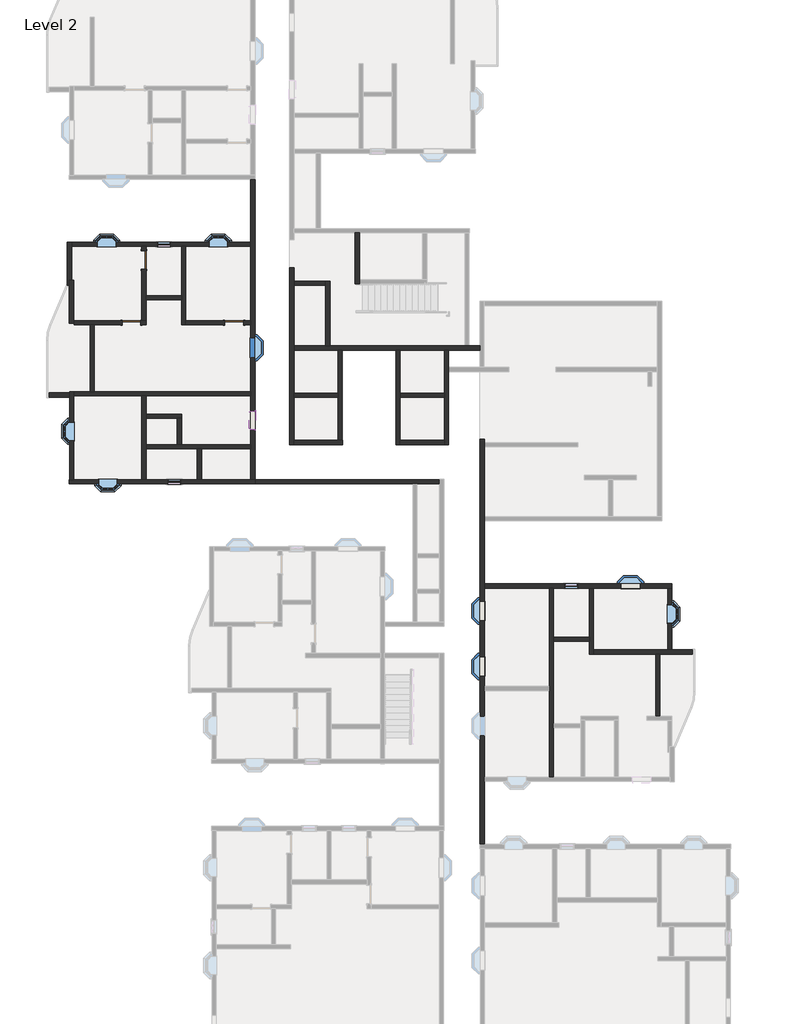
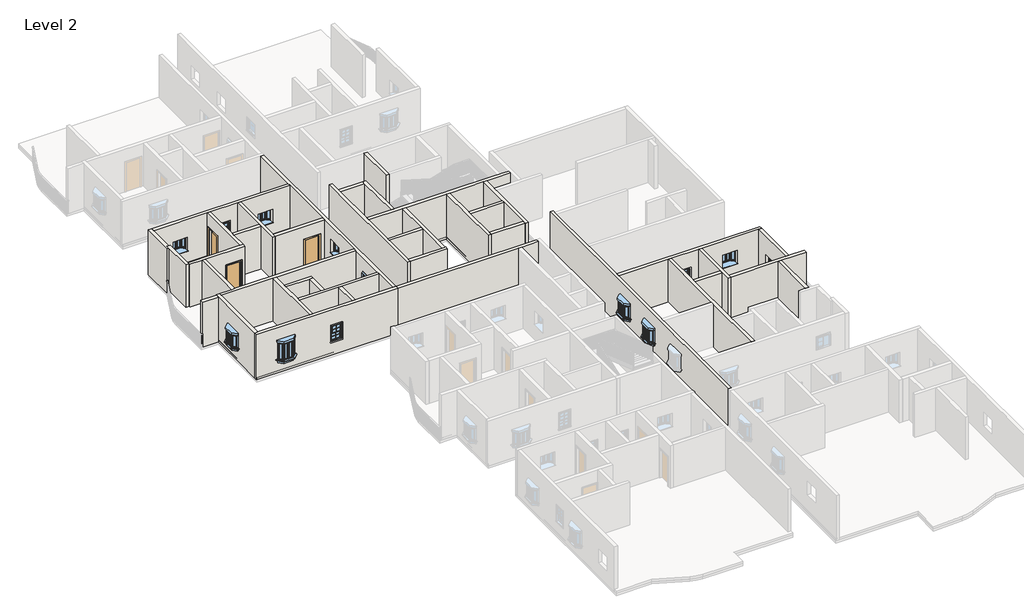
# One storey, part 3 of 14: 40 walls, 13 windows, 3 doors.
"""IFC4 building model written with IfcOpenShell, lengths in millimetres."""

from ifc_helpers import new_model, si_unit, frame, origin, place, context, project, spatial, polyline, outline, extrude, faceted_brep, transform, mapped, element, save
from components import door_54dd4da4, window_910x1210mm_154f9356, window_910x910mm_67ef725a, window_8debb0fa, windows_sgl_w_glazing_bars_910x910mm_256712d0

model = new_model("IFC4")

# Units and contexts
model_context = context("Model", 3, world=origin())
ifc_project = project(units=[si_unit("LENGTHUNIT", "METRE", prefix="MILLI")], contexts=[model_context])

# Site, building, storey
site = spatial("IfcSite", under=ifc_project)
building = spatial("IfcBuilding", under=site)
storey = spatial("IfcBuildingStorey", under=building, Name="Level 2", Elevation=3048.0)

# Doors
placement = place(None, origin())
door_shape = door_54dd4da4(model_context)
element("IfcDoor", 1, ObjectType="Single-Flush : 36\" x 84\"", at=placement, inside=storey, context=model_context, shape_type="MappedRepresentation", body=[
    mapped(door_shape, transform((-11210.3891351, 10605.7083494, 3048.0), x_axis=(1.0, 0.0, 0.0), y_axis=(0.0, 1.0, 0.0), z_axis=(0.0, 0.0, 1.0))),
])
element("IfcDoor", 2, ObjectType="Single-Flush : 36\" x 84\"", at=placement, inside=storey, context=model_context, shape_type="MappedRepresentation", body=[
    mapped(door_shape, transform((-15610.9391351, 13672.7583494, 3048.0), x_axis=(0.0, -1.0, 0.0), y_axis=(1.0, 0.0, 0.0), z_axis=(0.0, 0.0, 1.0))),
])
element("IfcDoor", 3, ObjectType="Single-Flush : 36\" x 84\"", at=placement, inside=storey, context=model_context, shape_type="MappedRepresentation", body=[
    mapped(door_shape, transform((-16220.5391351, 10605.7083494, 3048.0), x_axis=(1.0, 0.0, 0.0), y_axis=(0.0, 1.0, 0.0), z_axis=(0.0, 0.0, 1.0))),
])

# Walls
element("IfcWall", 4, ObjectType="4.5\" p", at=placement, inside=storey, context=model_context, shape_type="Brep", body=[
    faceted_brep([(-15509.3391351, 4456.3873146, 3048.0), (-13007.4391351, 4456.3873146, 3048.0), (-12804.2391351, 4456.3873146, 3048.0), (-10397.5891351, 4456.3873146, 3048.0), (-10397.5891351, 4456.3873146, 6096.0), (-12804.2391351, 4456.3873146, 6096.0), (-13007.4391351, 4456.3873146, 6096.0), (-15509.3391351, 4456.3873146, 6096.0), (-15509.3391351, 4659.5873146, 3048.0), (-15509.3391351, 4659.5873146, 6096.0), (-13985.3391351, 4659.5873146, 6096.0), (-13782.1391351, 4659.5873146, 6096.0), (-10397.5891351, 4659.5873146, 6096.0), (-10397.5891351, 4659.5873146, 3048.0), (-13782.1391351, 4659.5873146, 3048.0), (-13985.3391351, 4659.5873146, 3048.0)], [[[0, 1, 2, 3, 4, 5, 6, 7]], [[8, 9, 10, 11, 12, 13, 14, 15]], [[3, 2, 1, 0, 8, 15, 14, 13]], [[7, 6, 5, 4, 12, 11, 10, 9]], [[4, 3, 13, 12]], [[0, 7, 9, 8]]]),
])
element("IfcWall", 5, ObjectType="4.5\" p", at=placement, inside=storey, context=model_context, shape_type="SweptSolid", body=[
    extrude(outline(polyline([(-13007.4391351, 2953.9583494), (-13007.4391351, 4456.3873146), (-12804.2391351, 4456.3873146), (-12804.2391351, 2953.9583494), (-13007.4391351, 2953.9583494)])), frame((0.0, 0.0, 3048.0), z_axis=(0.0, 0.0, 1.0), x_axis=(1.0, 0.0, 0.0)), (0.0, 0.0, 1.0), 3048.0),
])
element("IfcWall", 6, ObjectType="4.5\" p", at=placement, inside=storey, context=model_context, shape_type="Brep", body=[
    faceted_brep([(-15509.3391351, 5953.2975261, 3048.0), (-13985.3391351, 5953.2975261, 3048.0), (-13782.1391351, 5953.2975261, 3048.0), (-13782.1391351, 5953.2975261, 6096.0), (-13985.3391351, 5953.2975261, 6096.0), (-15509.3391351, 5953.2975261, 6096.0), (-15509.3391351, 6156.4975261, 3048.0), (-15509.3391351, 6156.4975261, 6096.0), (-13782.1391351, 6156.4975261, 6096.0), (-13782.1391351, 6156.4975261, 3048.0)], [[[0, 1, 2, 3, 4, 5]], [[6, 7, 8, 9]], [[2, 1, 0, 6, 9]], [[5, 4, 3, 8, 7]], [[0, 5, 7, 6]], [[3, 2, 9, 8]]]),
])
element("IfcWall", 7, ObjectType="4.5\" p", at=placement, inside=storey, context=model_context, shape_type="SweptSolid", body=[
    extrude(outline(polyline([(-13985.3391351, 4659.5873146), (-13985.3391351, 5953.2975261), (-13782.1391351, 5953.2975261), (-13782.1391351, 4659.5873146), (-13985.3391351, 4659.5873146)])), frame((0.0, 0.0, 3048.0), z_axis=(0.0, 0.0, 1.0), x_axis=(1.0, 0.0, 0.0)), (0.0, 0.0, 1.0), 3048.0),
])
element("IfcWall", 8, ObjectType="4.5\" p", at=placement, inside=storey, context=model_context, shape_type="Brep", body=[
    faceted_brep([(-15712.5391351, 13215.5583494, 5181.6), (-15712.5391351, 13215.5583494, 3048.0), (-15712.5391351, 10707.3083494, 3048.0), (-15712.5391351, 10707.3083494, 6096.0), (-15712.5391351, 14333.1583494, 6096.0), (-15712.5391351, 14333.1583494, 3048.0), (-15712.5391351, 14129.9583494, 3048.0), (-15712.5391351, 14129.9583494, 5181.6), (-15509.3391351, 10707.3083494, 3048.0), (-15509.3391351, 11723.3083494, 3048.0), (-15509.3391351, 11926.5083494, 3048.0), (-15509.3391351, 13215.5583494, 3048.0), (-15509.3391351, 13215.5583494, 5181.6), (-15509.3391351, 14129.9583494, 5181.6), (-15509.3391351, 14129.9583494, 3048.0), (-15509.3391351, 14333.1583494, 3048.0), (-15509.3391351, 14333.1583494, 6096.0), (-15509.3391351, 11926.5083494, 6096.0), (-15509.3391351, 11723.3083494, 6096.0), (-15509.3391351, 10707.3083494, 6096.0)], [[[0, 1, 2, 3, 4, 5, 6, 7]], [[8, 9, 10, 11, 12, 13, 14, 15, 16, 17, 18, 19]], [[6, 5, 15, 14]], [[2, 1, 11, 10, 9, 8]], [[4, 3, 19, 18, 17, 16]], [[3, 2, 8, 19]], [[5, 4, 16, 15]], [[12, 11, 1, 0]], [[13, 12, 0, 7]], [[14, 13, 7, 6]]]),
])
element("IfcWall", 9, ObjectType="4.5\" p", at=placement, inside=storey, context=model_context, shape_type="Brep", body=[
    faceted_brep([(-13769.4391351, 14333.1583494, 3048.0), (-13769.4391351, 11926.5083494, 3048.0), (-13769.4391351, 11723.3083494, 3048.0), (-13769.4391351, 10504.1083494, 3048.0), (-13769.4391351, 10504.1083494, 6096.0), (-13769.4391351, 11723.3083494, 6096.0), (-13769.4391351, 11926.5083494, 6096.0), (-13769.4391351, 14333.1583494, 6096.0), (-13566.2391351, 14333.1583494, 3048.0), (-13566.2391351, 14333.1583494, 6096.0), (-13566.2391351, 10707.3083494, 6096.0), (-13566.2391351, 10504.1083494, 6096.0), (-13566.2391351, 10504.1083494, 3048.0), (-13566.2391351, 10707.3083494, 3048.0)], [[[0, 1, 2, 3, 4, 5, 6, 7]], [[8, 9, 10, 11, 12, 13]], [[3, 2, 1, 0, 8, 13, 12]], [[7, 6, 5, 4, 11, 10, 9]], [[0, 7, 9, 8]], [[4, 3, 12, 11]]]),
])
element("IfcWall", 10, ObjectType="4.5\" p", at=placement, inside=storey, context=model_context, shape_type="SweptSolid", body=[
    extrude(outline(polyline([(5181.6, -10753.1891351), (3048.0, -10753.1891351), (3048.0, -10397.5891351), (6096.0, -10397.5891351), (6096.0, -13566.2391351), (3048.0, -13566.2391351), (3048.0, -11667.5891351), (5181.6, -11667.5891351), (5181.6, -10753.1891351)])), frame((0.0, 10504.1083494, 0.0), z_axis=(0.0, 1.0, 0.0), x_axis=(0.0, 0.0, 1.0)), (0.0, 0.0, 1.0), 203.2),
])
element("IfcWall", 11, ObjectType="4.5\" p", at=placement, inside=storey, context=model_context, shape_type="SweptSolid", body=[
    extrude(outline(polyline([(-13769.4391351, 11723.3083494), (-15509.3391351, 11723.3083494), (-15509.3391351, 11926.5083494), (-13769.4391351, 11926.5083494), (-13769.4391351, 11723.3083494)])), frame((0.0, 0.0, 3048.0), z_axis=(0.0, 0.0, 1.0), x_axis=(1.0, 0.0, 0.0)), (0.0, 0.0, 1.0), 3048.0),
])
element("IfcWall", 12, ObjectType="4.5\" p", at=placement, inside=storey, context=model_context, shape_type="SweptSolid", body=[
    extrude(outline(polyline([(-6739.9891351, 12429.8715905), (-8289.3891351, 12429.8715905), (-8289.3891351, 12633.0715905), (-6739.9891351, 12633.0715905), (-6739.9891351, 12429.8715905)])), frame((0.0, 0.0, 3048.0), z_axis=(0.0, 0.0, 1.0), x_axis=(1.0, 0.0, 0.0)), (0.0, 0.0, 1.0), 3048.0),
])
element("IfcWall", 13, ObjectType="4.5\" p", at=placement, inside=storey, context=model_context, shape_type="SweptSolid", body=[
    extrude(outline(polyline([(-6130.3891351, 6970.2449943), (-8289.3891351, 6970.2449943), (-8289.3891351, 7173.4449943), (-6130.3891351, 7173.4449943), (-6130.3891351, 6970.2449943)])), frame((0.0, 0.0, 3048.0), z_axis=(0.0, 0.0, 1.0), x_axis=(1.0, 0.0, 0.0)), (0.0, 0.0, 1.0), 3048.0),
])
element("IfcWall", 14, ObjectType="4.5\" p", at=placement, inside=storey, context=model_context, shape_type="SweptSolid", body=[
    extrude(outline(polyline([(-948.7891351, 6970.2449943), (-3107.7891351, 6970.2449943), (-3107.7891351, 7173.4449943), (-948.7891351, 7173.4449943), (-948.7891351, 6970.2449943)])), frame((0.0, 0.0, 3048.0), z_axis=(0.0, 0.0, 1.0), x_axis=(1.0, 0.0, 0.0)), (0.0, 0.0, 1.0), 3048.0),
])
element("IfcWall", 15, ObjectType="4.5\" p", at=placement, inside=storey, context=model_context, shape_type="Brep", body=[
    faceted_brep([(-5298.5391351, 14988.9215905, 3048.0), (-5298.5391351, 12506.0715905, 3048.0), (-5298.5391351, 12506.0715905, 6096.0), (-5298.5391351, 14988.9215905, 6096.0), (-5095.3391351, 14988.9215905, 3048.0), (-5095.3391351, 14988.9215905, 6096.0), (-5095.3391351, 12709.2715905, 6096.0), (-5095.3391351, 12506.0715905, 6096.0), (-5095.3391351, 12506.0715905, 3048.0), (-5095.3391351, 12709.2715905, 3048.0)], [[[0, 1, 2, 3]], [[4, 5, 6, 7, 8, 9]], [[1, 0, 4, 9, 8]], [[3, 2, 7, 6, 5]], [[0, 3, 5, 4]], [[2, 1, 8, 7]]]),
])
element("IfcWall", 16, ObjectType="4.5\" p", at=placement, inside=storey, context=model_context, shape_type="SweptSolid", body=[
    extrude(outline(polyline([(-948.7891351, 4665.1949943), (-3107.7891351, 4665.1949943), (-3107.7891351, 4868.3949943), (-948.7891351, 4868.3949943), (-948.7891351, 4665.1949943)])), frame((0.0, 0.0, 3048.0), z_axis=(0.0, 0.0, 1.0), x_axis=(1.0, 0.0, 0.0)), (0.0, 0.0, 1.0), 3048.0),
])
element("IfcWall", 17, ObjectType="4.5\" p", at=placement, inside=storey, context=model_context, shape_type="Brep", body=[
    faceted_brep([(4184.4880523, -2336.4042694, 3048.0), (4184.4880523, -7130.6542694, 3048.0), (4184.4880523, -7333.8542694, 3048.0), (4184.4880523, -11556.6042694, 3048.0), (4184.4880523, -11556.6042694, 6096.0), (4184.4880523, -7333.8542694, 6096.0), (4184.4880523, -7130.6542694, 6096.0), (4184.4880523, -2336.4042694, 6096.0), (4387.6880523, -2336.4042694, 3048.0), (4387.6880523, -2336.4042694, 6096.0), (4387.6880523, -4736.7042694, 6096.0), (4387.6880523, -4939.9042694, 6096.0), (4387.6880523, -8959.4542694, 6096.0), (4387.6880523, -9162.6542694, 6096.0), (4387.6880523, -11556.6042694, 6096.0), (4387.6880523, -11556.6042694, 3048.0), (4387.6880523, -9162.6542694, 3048.0), (4387.6880523, -8959.4542694, 3048.0), (4387.6880523, -4939.9042694, 3048.0), (4387.6880523, -4736.7042694, 3048.0)], [[[0, 1, 2, 3, 4, 5, 6, 7]], [[8, 9, 10, 11, 12, 13, 14, 15, 16, 17, 18, 19]], [[3, 2, 1, 0, 8, 19, 18, 17, 16, 15]], [[7, 6, 5, 4, 14, 13, 12, 11, 10, 9]], [[4, 3, 15, 14]], [[0, 7, 9, 8]]]),
])
element("IfcWall", 18, ObjectType="4.5\" p", at=placement, inside=storey, context=model_context, shape_type="Brep", body=[
    faceted_brep([(803.8108649, 4915.2957306, 3048.0), (803.8108649, -14845.9042694, 3048.0), (803.8108649, -14845.9042694, 6096.0), (803.8108649, 4915.2957306, 6096.0), (803.8108649, -9516.0542694, 5158.0), (803.8108649, -9516.0542694, 4248.0), (803.8108649, -8606.0542694, 4248.0), (803.8108649, -8606.0542694, 5158.0), (803.8108649, -3909.0042694, 5158.0), (803.8108649, -3909.0042694, 4248.0), (803.8108649, -2999.0042694, 4248.0), (803.8108649, -2999.0042694, 5158.0), (803.8108649, -6620.4542694, 5158.0), (803.8108649, -6620.4542694, 4248.0), (803.8108649, -5710.4542694, 4248.0), (803.8108649, -5710.4542694, 5158.0), (1007.0108649, 4915.2957306, 3048.0), (1007.0108649, 4915.2957306, 6096.0), (1007.0108649, 4754.0949943, 6096.0), (1007.0108649, 4550.8949943, 6096.0), (1007.0108649, 1143.3957306, 6096.0), (1007.0108649, 940.1957306, 6096.0), (1007.0108649, -2133.2042694, 6096.0), (1007.0108649, -2336.4042694, 6096.0), (1007.0108649, -7130.6542694, 6096.0), (1007.0108649, -7333.8542694, 6096.0), (1007.0108649, -11556.6042694, 6096.0), (1007.0108649, -11759.8042694, 6096.0), (1007.0108649, -14845.9042694, 6096.0), (1007.0108649, -14845.9042694, 3048.0), (1007.0108649, -11759.8042694, 3048.0), (1007.0108649, -11556.6042694, 3048.0), (1007.0108649, -7333.8542694, 3048.0), (1007.0108649, -7130.6542694, 3048.0), (1007.0108649, -2336.4042694, 3048.0), (1007.0108649, -2133.2042694, 3048.0), (1007.0108649, 940.1957306, 3048.0), (1007.0108649, 1143.3957306, 3048.0), (1007.0108649, 4550.8949943, 3048.0), (1007.0108649, 4754.0949943, 3048.0), (1007.0108649, -9516.0542694, 5158.0), (1007.0108649, -8606.0542694, 5158.0), (1007.0108649, -8606.0542694, 4248.0), (1007.0108649, -9516.0542694, 4248.0), (1007.0108649, -3909.0042694, 5158.0), (1007.0108649, -2999.0042694, 5158.0), (1007.0108649, -2999.0042694, 4248.0), (1007.0108649, -3909.0042694, 4248.0), (1007.0108649, -6620.4542694, 5158.0), (1007.0108649, -5710.4542694, 5158.0), (1007.0108649, -5710.4542694, 4248.0), (1007.0108649, -6620.4542694, 4248.0)], [[[0, 1, 2, 3], [4, 5, 6, 7], [8, 9, 10, 11], [12, 13, 14, 15]], [[16, 17, 18, 19, 20, 21, 22, 23, 24, 25, 26, 27, 28, 29, 30, 31, 32, 33, 34, 35, 36, 37, 38, 39], [40, 41, 42, 43], [44, 45, 46, 47], [48, 49, 50, 51]], [[1, 0, 16, 39, 38, 37, 36, 35, 34, 33, 32, 31, 30, 29]], [[3, 2, 28, 27, 26, 25, 24, 23, 22, 21, 20, 19, 18, 17]], [[0, 3, 17, 16]], [[2, 1, 29, 28]], [[5, 4, 40, 43]], [[6, 5, 43, 42]], [[7, 6, 42, 41]], [[4, 7, 41, 40]], [[9, 8, 44, 47]], [[10, 9, 47, 46]], [[11, 10, 46, 45]], [[8, 11, 45, 44]], [[13, 12, 48, 51]], [[14, 13, 51, 50]], [[15, 14, 50, 49]], [[12, 15, 49, 48]]]),
])
element("IfcWall", 19, ObjectType="4.5\" p", at=placement, inside=storey, context=model_context, shape_type="SweptSolid", body=[
    extrude(outline(polyline([(6127.5880523, -4939.9042694), (4387.6880523, -4939.9042694), (4387.6880523, -4736.7042694), (6127.5880523, -4736.7042694), (6127.5880523, -4939.9042694)])), frame((0.0, 0.0, 3048.0), z_axis=(0.0, 0.0, 1.0), x_axis=(1.0, 0.0, 0.0)), (0.0, 0.0, 1.0), 3048.0),
])
element("IfcWall", 20, ObjectType="4.5\" p", at=placement, inside=storey, context=model_context, shape_type="Brep", body=[
    faceted_brep([(6127.5880523, -2336.4042694, 3048.0), (6127.5880523, -4736.7042694, 3048.0), (6127.5880523, -4939.9042694, 3048.0), (6127.5880523, -5555.8542694, 3048.0), (6127.5880523, -5555.8542694, 6096.0), (6127.5880523, -4939.9042694, 6096.0), (6127.5880523, -4736.7042694, 6096.0), (6127.5880523, -2336.4042694, 6096.0), (6330.7880523, -2336.4042694, 3048.0), (6330.7880523, -2336.4042694, 6096.0), (6330.7880523, -5352.6542694, 6096.0), (6330.7880523, -5555.8542694, 6096.0), (6330.7880523, -5555.8542694, 3048.0), (6330.7880523, -5352.6542694, 3048.0)], [[[0, 1, 2, 3, 4, 5, 6, 7]], [[8, 9, 10, 11, 12, 13]], [[3, 2, 1, 0, 8, 13, 12]], [[7, 6, 5, 4, 11, 10, 9]], [[0, 7, 9, 8]], [[4, 3, 12, 11]]]),
])
element("IfcWall", 21, ObjectType="4.5\" p", at=placement, inside=storey, context=model_context, shape_type="Brep", body=[
    faceted_brep([(6330.7880523, -5555.8542694, 3048.0), (9371.2322031, -5555.8542694, 3048.0), (9574.4322031, -5555.8542694, 3048.0), (11163.1380523, -5555.8542694, 3048.0), (11163.1380523, -5555.8542694, 6096.0), (9574.4322031, -5555.8542694, 6096.0), (9371.2322031, -5555.8542694, 6096.0), (6330.7880523, -5555.8542694, 6096.0), (6330.7880523, -5352.6542694, 3048.0), (6330.7880523, -5352.6542694, 6096.0), (9956.6380523, -5352.6542694, 6096.0), (10159.8380523, -5352.6542694, 6096.0), (11163.1380523, -5352.6542694, 6096.0), (11163.1380523, -5352.6542694, 3048.0), (10159.8380523, -5352.6542694, 3048.0), (9956.6380523, -5352.6542694, 3048.0)], [[[0, 1, 2, 3, 4, 5, 6, 7]], [[8, 9, 10, 11, 12, 13, 14, 15]], [[3, 2, 1, 0, 8, 15, 14, 13]], [[4, 3, 13, 12]], [[7, 6, 5, 4, 12, 11, 10, 9]], [[0, 7, 9, 8]]]),
])
element("IfcWall", 22, ObjectType="4.5\" p", at=placement, inside=storey, context=model_context, shape_type="SweptSolid", body=[
    extrude(outline(polyline([(9371.2322031, -8578.4542694), (9371.2322031, -5555.8542694), (9574.4322031, -5555.8542694), (9574.4322031, -8578.4542694), (9371.2322031, -8578.4542694)])), frame((0.0, 0.0, 3048.0), z_axis=(0.0, 0.0, 1.0), x_axis=(1.0, 0.0, 0.0)), (0.0, 0.0, 1.0), 3048.0),
])
element("IfcWall", 23, ObjectType="9\"", at=placement, inside=storey, context=model_context, shape_type="Brep", body=[
    faceted_brep([(-10181.6891351, 2953.9583494, 3048.0), (-10194.3891351, 2953.9583494, 3048.0), (-10397.5891351, 2953.9583494, 3048.0), (-12804.2391351, 2953.9583494, 3048.0), (-13007.4391351, 2953.9583494, 3048.0), (-15509.3391351, 2953.9583494, 3048.0), (-15712.5391351, 2953.9583494, 3048.0), (-19033.5891351, 2953.9583494, 3048.0), (-19236.7891351, 2953.9583494, 3048.0), (-19249.4891351, 2953.9583494, 3048.0), (-19249.4891351, 2953.9583494, 6096.0), (-19236.7891351, 2953.9583494, 6096.0), (-19033.5891351, 2953.9583494, 6096.0), (-15712.5391351, 2953.9583494, 6096.0), (-15509.3391351, 2953.9583494, 6096.0), (-13007.4391351, 2953.9583494, 6096.0), (-12804.2391351, 2953.9583494, 6096.0), (-10397.5891351, 2953.9583494, 6096.0), (-10194.3891351, 2953.9583494, 6096.0), (-10181.6891351, 2953.9583494, 6096.0), (-13794.8391351, 2953.9583494, 5029.2), (-14455.2391351, 2953.9583494, 5029.2), (-14455.2391351, 2953.9583494, 3962.4), (-13794.8391351, 2953.9583494, 3962.4), (-16918.0641351, 2953.9583494, 5172.4), (-17828.0641351, 2953.9583494, 5172.4), (-17828.0641351, 2953.9583494, 3962.4), (-16918.0641351, 2953.9583494, 3962.4), (-10181.6891351, 2750.7583494, 3048.0), (-10181.6891351, 2750.7583494, 6096.0), (-19249.4891351, 2750.7583494, 6096.0), (-19249.4891351, 2750.7583494, 3048.0), (-13794.8391351, 2750.7583494, 5029.2), (-13794.8391351, 2750.7583494, 3962.4), (-14455.2391351, 2750.7583494, 3962.4), (-14455.2391351, 2750.7583494, 5029.2), (-16918.0641351, 2750.7583494, 5172.4), (-16918.0641351, 2750.7583494, 3962.4), (-17828.0641351, 2750.7583494, 3962.4), (-17828.0641351, 2750.7583494, 5172.4)], [[[0, 1, 2, 3, 4, 5, 6, 7, 8, 9, 10, 11, 12, 13, 14, 15, 16, 17, 18, 19], [20, 21, 22, 23], [24, 25, 26, 27]], [[28, 29, 30, 31], [32, 33, 34, 35], [36, 37, 38, 39]], [[9, 8, 7, 6, 5, 4, 3, 2, 1, 0, 28, 31]], [[10, 9, 31, 30]], [[19, 18, 17, 16, 15, 14, 13, 12, 11, 10, 30, 29]], [[0, 19, 29, 28]], [[33, 32, 20, 23]], [[34, 33, 23, 22]], [[35, 34, 22, 21]], [[32, 35, 21, 20]], [[37, 36, 24, 27]], [[38, 37, 27, 26]], [[39, 38, 26, 25]], [[36, 39, 25, 24]]]),
])
element("IfcWall", 24, ObjectType="9\"", at=placement, inside=storey, context=model_context, shape_type="Brep", body=[
    faceted_brep([(-19033.5891351, 2953.9583494, 3048.0), (-19033.5891351, 7037.0083494, 3048.0), (-19033.5891351, 7240.2083494, 3048.0), (-19033.5891351, 7240.2083494, 6096.0), (-19033.5891351, 7037.0083494, 6096.0), (-19033.5891351, 2953.9583494, 6096.0), (-19033.5891351, 4854.8083494, 4872.4), (-19033.5891351, 5764.8083494, 4872.4), (-19033.5891351, 5764.8083494, 3962.4), (-19033.5891351, 4854.8083494, 3962.4), (-19236.7891351, 2953.9583494, 3048.0), (-19236.7891351, 2953.9583494, 6096.0), (-19236.7891351, 7240.2083494, 6096.0), (-19236.7891351, 7240.2083494, 3048.0), (-19236.7891351, 4854.8083494, 4872.4), (-19236.7891351, 4854.8083494, 3962.4), (-19236.7891351, 5764.8083494, 3962.4), (-19236.7891351, 5764.8083494, 4872.4)], [[[0, 1, 2, 3, 4, 5], [6, 7, 8, 9]], [[10, 11, 12, 13], [14, 15, 16, 17]], [[2, 1, 0, 10, 13]], [[5, 4, 3, 12, 11]], [[0, 5, 11, 10]], [[3, 2, 13, 12]], [[15, 14, 6, 9]], [[16, 15, 9, 8]], [[17, 16, 8, 7]], [[14, 17, 7, 6]]]),
])
element("IfcWall", 25, ObjectType="9\"", at=placement, inside=storey, context=model_context, shape_type="Brep", body=[
    faceted_brep([(-10194.3891351, 2953.9583494, 3048.0), (-10194.3891351, 17597.0583494, 3048.0), (-10194.3891351, 17597.0583494, 6096.0), (-10194.3891351, 2953.9583494, 6096.0), (-10194.3891351, 9841.5083494, 5158.0), (-10194.3891351, 9841.5083494, 4248.0), (-10194.3891351, 8931.5083494, 4248.0), (-10194.3891351, 8931.5083494, 5158.0), (-10194.3891351, 5393.297832, 5158.0), (-10194.3891351, 6303.297832, 5158.0), (-10194.3891351, 6303.297832, 4248.0), (-10194.3891351, 5393.297832, 4248.0), (-10397.5891351, 2953.9583494, 3048.0), (-10397.5891351, 2953.9583494, 6096.0), (-10397.5891351, 4456.3873146, 6096.0), (-10397.5891351, 4659.5873146, 6096.0), (-10397.5891351, 7037.0083494, 6096.0), (-10397.5891351, 7240.2083494, 6096.0), (-10397.5891351, 10504.1083494, 6096.0), (-10397.5891351, 10707.3083494, 6096.0), (-10397.5891351, 14333.1583494, 6096.0), (-10397.5891351, 14536.3583494, 6096.0), (-10397.5891351, 17597.0583494, 6096.0), (-10397.5891351, 17597.0583494, 3048.0), (-10397.5891351, 14536.3583494, 3048.0), (-10397.5891351, 14333.1583494, 3048.0), (-10397.5891351, 10707.3083494, 3048.0), (-10397.5891351, 10504.1083494, 3048.0), (-10397.5891351, 7240.2083494, 3048.0), (-10397.5891351, 7037.0083494, 3048.0), (-10397.5891351, 4659.5873146, 3048.0), (-10397.5891351, 4456.3873146, 3048.0), (-10397.5891351, 9841.5083494, 5158.0), (-10397.5891351, 8931.5083494, 5158.0), (-10397.5891351, 8931.5083494, 4248.0), (-10397.5891351, 9841.5083494, 4248.0), (-10397.5891351, 5393.297832, 5158.0), (-10397.5891351, 5393.297832, 4248.0), (-10397.5891351, 6303.297832, 4248.0), (-10397.5891351, 6303.297832, 5158.0)], [[[0, 1, 2, 3], [4, 5, 6, 7], [8, 9, 10, 11]], [[12, 13, 14, 15, 16, 17, 18, 19, 20, 21, 22, 23, 24, 25, 26, 27, 28, 29, 30, 31], [32, 33, 34, 35], [36, 37, 38, 39]], [[1, 0, 12, 31, 30, 29, 28, 27, 26, 25, 24, 23]], [[2, 1, 23, 22]], [[3, 2, 22, 21, 20, 19, 18, 17, 16, 15, 14, 13]], [[0, 3, 13, 12]], [[5, 4, 32, 35]], [[6, 5, 35, 34]], [[7, 6, 34, 33]], [[4, 7, 33, 32]], [[37, 36, 8, 11]], [[38, 37, 11, 10]], [[39, 38, 10, 9]], [[36, 39, 9, 8]]]),
])
element("IfcWall", 26, ObjectType="9\"", at=placement, inside=storey, context=model_context, shape_type="SweptSolid", body=[
    extrude(outline(polyline([(-19249.4891351, 6979.8583494), (-20240.0891351, 6979.8583494), (-20240.0891351, 7183.0583494), (-19249.4891351, 7183.0583494), (-19249.4891351, 6979.8583494)])), frame((0.0, 0.0, 3048.0), z_axis=(0.0, 0.0, 1.0), x_axis=(1.0, 0.0, 0.0)), (0.0, 0.0, 1.0), 3048.0),
])
element("IfcWall", 27, ObjectType="9\"", at=placement, inside=storey, context=model_context, shape_type="Brep", body=[
    faceted_brep([(-19147.8891351, 12435.1858981, 3048.0), (-19147.8891351, 14333.1583494, 3048.0), (-19147.8891351, 14536.3583494, 3048.0), (-19147.8891351, 14549.0583494, 3048.0), (-19147.8891351, 14549.0583494, 6096.0), (-19147.8891351, 14536.3583494, 6096.0), (-19147.8891351, 14333.1583494, 6096.0), (-19147.8891351, 12435.1858981, 6096.0), (-19351.0891351, 12435.1858981, 3048.0), (-19351.0891351, 12435.1858981, 6096.0), (-19351.0891351, 14549.0583494, 6096.0), (-19351.0891351, 14549.0583494, 3048.0)], [[[0, 1, 2, 3, 4, 5, 6, 7]], [[8, 9, 10, 11]], [[3, 2, 1, 0, 8, 11]], [[4, 3, 11, 10]], [[7, 6, 5, 4, 10, 9]], [[0, 7, 9, 8]]]),
])
element("IfcWall", 28, ObjectType="9\"", at=placement, inside=storey, context=model_context, shape_type="Brep", body=[
    faceted_brep([(-19147.8891351, 14333.1583494, 3048.0), (-15712.5391351, 14333.1583494, 3048.0), (-15509.3391351, 14333.1583494, 3048.0), (-13769.4391351, 14333.1583494, 3048.0), (-13566.2391351, 14333.1583494, 3048.0), (-10397.5891351, 14333.1583494, 3048.0), (-10397.5891351, 14333.1583494, 6096.0), (-13566.2391351, 14333.1583494, 6096.0), (-13769.4391351, 14333.1583494, 6096.0), (-15509.3391351, 14333.1583494, 6096.0), (-15712.5391351, 14333.1583494, 6096.0), (-19147.8891351, 14333.1583494, 6096.0), (-17885.2141351, 14333.1583494, 4872.4), (-16975.2141351, 14333.1583494, 4872.4), (-16975.2141351, 14333.1583494, 3962.4), (-17885.2141351, 14333.1583494, 3962.4), (-12436.9141351, 14333.1583494, 4872.4), (-11526.9141351, 14333.1583494, 4872.4), (-11526.9141351, 14333.1583494, 3962.4), (-12436.9141351, 14333.1583494, 3962.4), (-14309.1891351, 14333.1583494, 5029.2), (-14309.1891351, 14333.1583494, 3962.4), (-14969.5891351, 14333.1583494, 3962.4), (-14969.5891351, 14333.1583494, 5029.2), (-19147.8891351, 14536.3583494, 3048.0), (-19147.8891351, 14536.3583494, 6096.0), (-10397.5891351, 14536.3583494, 6096.0), (-10397.5891351, 14536.3583494, 3048.0), (-17885.2141351, 14536.3583494, 4872.4), (-17885.2141351, 14536.3583494, 3962.4), (-16975.2141351, 14536.3583494, 3962.4), (-16975.2141351, 14536.3583494, 4872.4), (-12436.9141351, 14536.3583494, 4872.4), (-12436.9141351, 14536.3583494, 3962.4), (-11526.9141351, 14536.3583494, 3962.4), (-11526.9141351, 14536.3583494, 4872.4), (-14309.1891351, 14536.3583494, 5029.2), (-14969.5891351, 14536.3583494, 5029.2), (-14969.5891351, 14536.3583494, 3962.4), (-14309.1891351, 14536.3583494, 3962.4)], [[[0, 1, 2, 3, 4, 5, 6, 7, 8, 9, 10, 11], [12, 13, 14, 15], [16, 17, 18, 19], [20, 21, 22, 23]], [[24, 25, 26, 27], [28, 29, 30, 31], [32, 33, 34, 35], [36, 37, 38, 39]], [[5, 4, 3, 2, 1, 0, 24, 27]], [[11, 10, 9, 8, 7, 6, 26, 25]], [[6, 5, 27, 26]], [[0, 11, 25, 24]], [[29, 28, 12, 15]], [[30, 29, 15, 14]], [[31, 30, 14, 13]], [[28, 31, 13, 12]], [[33, 32, 16, 19]], [[34, 33, 19, 18]], [[35, 34, 18, 17]], [[32, 35, 17, 16]], [[21, 20, 36, 39]], [[22, 21, 39, 38]], [[23, 22, 38, 37]], [[20, 23, 37, 36]]]),
])
element("IfcWall", 29, ObjectType="9\"", at=placement, inside=storey, context=model_context, shape_type="SweptSolid", body=[
    extrude(outline(polyline([(-19249.4891351, 10585.5474528), (-19249.4891351, 12672.4473407), (-19046.2891351, 12672.4473407), (-19046.2891351, 10585.5474528), (-19249.4891351, 10585.5474528)])), frame((0.0, 0.0, 3048.0), z_axis=(0.0, 0.0, 1.0), x_axis=(1.0, 0.0, 0.0)), (0.0, 0.0, 1.0), 3048.0),
])
element("IfcWall", 30, ObjectType="9\" w", at=placement, inside=storey, context=model_context, shape_type="Brep", body=[
    faceted_brep([(-1177.3891351, 2953.9583494, 3048.0), (-10181.6891351, 2953.9583494, 3048.0), (-10181.6891351, 2953.9583494, 6096.0), (-1177.3891351, 2953.9583494, 6096.0), (-1177.3891351, 2750.7583494, 3048.0), (-1177.3891351, 2750.7583494, 6096.0), (-2269.5891351, 2750.7583494, 6096.0), (-2472.7891351, 2750.7583494, 6096.0), (-10181.6891351, 2750.7583494, 6096.0), (-10181.6891351, 2750.7583494, 3048.0), (-2472.7891351, 2750.7583494, 3048.0), (-2269.5891351, 2750.7583494, 3048.0)], [[[0, 1, 2, 3]], [[4, 5, 6, 7, 8, 9, 10, 11]], [[1, 0, 4, 11, 10, 9]], [[2, 1, 9, 8]], [[3, 2, 8, 7, 6, 5]], [[0, 3, 5, 4]]]),
])
element("IfcWall", 31, ObjectType="9\" w", at=placement, inside=storey, context=model_context, shape_type="Brep", body=[
    faceted_brep([(-15763.3391351, 10504.1083494, 5181.6), (-15763.3391351, 10504.1083494, 3048.0), (-15509.3391351, 10504.1083494, 3048.0), (-15509.3391351, 10504.1083494, 6096.0), (-18042.9891351, 10504.1083494, 6096.0), (-18246.1891351, 10504.1083494, 6096.0), (-19027.2391351, 10504.1083494, 6096.0), (-19027.2391351, 10504.1083494, 3048.0), (-18246.1891351, 10504.1083494, 3048.0), (-18042.9891351, 10504.1083494, 3048.0), (-16677.7391351, 10504.1083494, 3048.0), (-16677.7391351, 10504.1083494, 5181.6), (-15509.3391351, 10707.3083494, 3048.0), (-15712.5391351, 10707.3083494, 3048.0), (-15763.3391351, 10707.3083494, 3048.0), (-15763.3391351, 10707.3083494, 5181.6), (-16677.7391351, 10707.3083494, 5181.6), (-16677.7391351, 10707.3083494, 3048.0), (-19027.2391351, 10707.3083494, 3048.0), (-19027.2391351, 10707.3083494, 6096.0), (-15712.5391351, 10707.3083494, 6096.0), (-15509.3391351, 10707.3083494, 6096.0)], [[[0, 1, 2, 3, 4, 5, 6, 7, 8, 9, 10, 11]], [[12, 13, 14, 15, 16, 17, 18, 19, 20, 21]], [[2, 1, 14, 13, 12]], [[10, 9, 8, 7, 18, 17]], [[6, 5, 4, 3, 21, 20, 19]], [[7, 6, 19, 18]], [[3, 2, 12, 21]], [[15, 14, 1, 0]], [[16, 15, 0, 11]], [[17, 16, 11, 10]]]),
])
element("IfcWall", 32, ObjectType="9\" w", at=placement, inside=storey, context=model_context, shape_type="SweptSolid", body=[
    extrude(outline(polyline([(-18246.1891351, 7240.2083494), (-18246.1891351, 10504.1083494), (-18042.9891351, 10504.1083494), (-18042.9891351, 7240.2083494), (-18246.1891351, 7240.2083494)])), frame((0.0, 0.0, 3048.0), z_axis=(0.0, 0.0, 1.0), x_axis=(1.0, 0.0, 0.0)), (0.0, 0.0, 1.0), 3048.0),
])
element("IfcWall", 33, ObjectType="9\" w", at=placement, inside=storey, context=model_context, shape_type="Brep", body=[
    faceted_brep([(-19033.5891351, 7037.0083494, 3048.0), (-15712.5391351, 7037.0083494, 3048.0), (-15509.3391351, 7037.0083494, 3048.0), (-10397.5891351, 7037.0083494, 3048.0), (-10397.5891351, 7037.0083494, 6096.0), (-15509.3391351, 7037.0083494, 6096.0), (-15712.5391351, 7037.0083494, 6096.0), (-19033.5891351, 7037.0083494, 6096.0), (-19033.5891351, 7240.2083494, 3048.0), (-19033.5891351, 7240.2083494, 6096.0), (-18246.1891351, 7240.2083494, 6096.0), (-18042.9891351, 7240.2083494, 6096.0), (-10397.5891351, 7240.2083494, 6096.0), (-10397.5891351, 7240.2083494, 3048.0), (-18042.9891351, 7240.2083494, 3048.0), (-18246.1891351, 7240.2083494, 3048.0)], [[[0, 1, 2, 3, 4, 5, 6, 7]], [[8, 9, 10, 11, 12, 13, 14, 15]], [[3, 2, 1, 0, 8, 15, 14, 13]], [[7, 6, 5, 4, 12, 11, 10, 9]], [[0, 7, 9, 8]], [[4, 3, 13, 12]]]),
])
element("IfcWall", 34, ObjectType="9\" w", at=placement, inside=storey, context=model_context, shape_type="Brep", body=[
    faceted_brep([(-15712.5391351, 7037.0083494, 3048.0), (-15712.5391351, 2953.9583494, 3048.0), (-15712.5391351, 2953.9583494, 6096.0), (-15712.5391351, 7037.0083494, 6096.0), (-15509.3391351, 7037.0083494, 3048.0), (-15509.3391351, 7037.0083494, 6096.0), (-15509.3391351, 6156.4975261, 6096.0), (-15509.3391351, 5953.2975261, 6096.0), (-15509.3391351, 4659.5873146, 6096.0), (-15509.3391351, 4456.3873146, 6096.0), (-15509.3391351, 2953.9583494, 6096.0), (-15509.3391351, 2953.9583494, 3048.0), (-15509.3391351, 4456.3873146, 3048.0), (-15509.3391351, 4659.5873146, 3048.0), (-15509.3391351, 5953.2975261, 3048.0), (-15509.3391351, 6156.4975261, 3048.0)], [[[0, 1, 2, 3]], [[4, 5, 6, 7, 8, 9, 10, 11, 12, 13, 14, 15]], [[1, 0, 4, 15, 14, 13, 12, 11]], [[3, 2, 10, 9, 8, 7, 6, 5]], [[2, 1, 11, 10]], [[0, 3, 5, 4]]]),
])
element("IfcWall", 35, ObjectType="9\" w", at=placement, inside=storey, context=model_context, shape_type="Brep", body=[
    faceted_brep([(-8492.5891351, 13295.1410318, 3048.0), (-8492.5891351, 4652.4949943, 3048.0), (-8492.5891351, 4652.4949943, 6096.0), (-8492.5891351, 13295.1410318, 6096.0), (-8289.3891351, 13295.1410318, 3048.0), (-8289.3891351, 13295.1410318, 6096.0), (-8289.3891351, 12633.0715905, 6096.0), (-8289.3891351, 12429.8715905, 6096.0), (-8289.3891351, 9478.4949943, 6096.0), (-8289.3891351, 9275.2949943, 6096.0), (-8289.3891351, 7173.4449943, 6096.0), (-8289.3891351, 6970.2449943, 6096.0), (-8289.3891351, 4868.3949943, 6096.0), (-8289.3891351, 4665.1949943, 6096.0), (-8289.3891351, 4652.4949943, 6096.0), (-8289.3891351, 4652.4949943, 3048.0), (-8289.3891351, 4665.1949943, 3048.0), (-8289.3891351, 4868.3949943, 3048.0), (-8289.3891351, 6970.2449943, 3048.0), (-8289.3891351, 7173.4449943, 3048.0), (-8289.3891351, 9275.2949943, 3048.0), (-8289.3891351, 9478.4949943, 3048.0), (-8289.3891351, 12429.8715905, 3048.0), (-8289.3891351, 12633.0715905, 3048.0)], [[[0, 1, 2, 3]], [[4, 5, 6, 7, 8, 9, 10, 11, 12, 13, 14, 15, 16, 17, 18, 19, 20, 21, 22, 23]], [[1, 0, 4, 23, 22, 21, 20, 19, 18, 17, 16, 15]], [[2, 1, 15, 14]], [[3, 2, 14, 13, 12, 11, 10, 9, 8, 7, 6, 5]], [[0, 3, 5, 4]]]),
])
element("IfcWall", 36, ObjectType="9\" w", at=placement, inside=storey, context=model_context, shape_type="Brep", body=[
    faceted_brep([(-8289.3891351, 4665.1949943, 3048.0), (-5914.4891351, 4665.1949943, 3048.0), (-5914.4891351, 4665.1949943, 6096.0), (-8289.3891351, 4665.1949943, 6096.0), (-8289.3891351, 4868.3949943, 3048.0), (-8289.3891351, 4868.3949943, 6096.0), (-6130.3891351, 4868.3949943, 6096.0), (-5927.1891351, 4868.3949943, 6096.0), (-5914.4891351, 4868.3949943, 6096.0), (-5914.4891351, 4868.3949943, 3048.0), (-5927.1891351, 4868.3949943, 3048.0), (-6130.3891351, 4868.3949943, 3048.0)], [[[0, 1, 2, 3]], [[4, 5, 6, 7, 8, 9, 10, 11]], [[1, 0, 4, 11, 10, 9]], [[2, 1, 9, 8]], [[3, 2, 8, 7, 6, 5]], [[0, 3, 5, 4]]]),
])
element("IfcWall", 37, ObjectType="9\" w", at=placement, inside=storey, context=model_context, shape_type="Brep", body=[
    faceted_brep([(-5927.1891351, 4868.3949943, 3048.0), (-5927.1891351, 9275.2949943, 3048.0), (-5927.1891351, 9275.2949943, 6096.0), (-5927.1891351, 4868.3949943, 6096.0), (-6130.3891351, 4868.3949943, 3048.0), (-6130.3891351, 4868.3949943, 6096.0), (-6130.3891351, 6970.2449943, 6096.0), (-6130.3891351, 7173.4449943, 6096.0), (-6130.3891351, 9275.2949943, 6096.0), (-6130.3891351, 9275.2949943, 3048.0), (-6130.3891351, 7173.4449943, 3048.0), (-6130.3891351, 6970.2449943, 3048.0)], [[[0, 1, 2, 3]], [[4, 5, 6, 7, 8, 9, 10, 11]], [[1, 0, 4, 11, 10, 9]], [[3, 2, 8, 7, 6, 5]], [[0, 3, 5, 4]], [[2, 1, 9, 8]]]),
])
element("IfcWall", 38, ObjectType="9\" w", at=placement, inside=storey, context=model_context, shape_type="Brep", body=[
    faceted_brep([(-8289.3891351, 9275.2949943, 3048.0), (-6130.3891351, 9275.2949943, 3048.0), (-5927.1891351, 9275.2949943, 3048.0), (-3310.9891351, 9275.2949943, 3048.0), (-3107.7891351, 9275.2949943, 3048.0), (-948.7891351, 9275.2949943, 3048.0), (-745.5891351, 9275.2949943, 3048.0), (793.5880523, 9275.2949943, 3048.0), (793.5880523, 9275.2949943, 6096.0), (-745.5891351, 9275.2949943, 6096.0), (-948.7891351, 9275.2949943, 6096.0), (-3107.7891351, 9275.2949943, 6096.0), (-3310.9891351, 9275.2949943, 6096.0), (-5927.1891351, 9275.2949943, 6096.0), (-6130.3891351, 9275.2949943, 6096.0), (-8289.3891351, 9275.2949943, 6096.0), (-8289.3891351, 9478.4949943, 3048.0), (-8289.3891351, 9478.4949943, 6096.0), (-6739.9891351, 9478.4949943, 6096.0), (-6536.7891351, 9478.4949943, 6096.0), (54.5108649, 9478.4949943, 6096.0), (257.7108649, 9478.4949943, 6096.0), (793.5880523, 9478.4949943, 6096.0), (793.5880523, 9478.4949943, 3048.0), (257.7108649, 9478.4949943, 3048.0), (54.5108649, 9478.4949943, 3048.0), (-6536.7891351, 9478.4949943, 3048.0), (-6739.9891351, 9478.4949943, 3048.0)], [[[0, 1, 2, 3, 4, 5, 6, 7, 8, 9, 10, 11, 12, 13, 14, 15]], [[16, 17, 18, 19, 20, 21, 22, 23, 24, 25, 26, 27]], [[7, 6, 5, 4, 3, 2, 1, 0, 16, 27, 26, 25, 24, 23]], [[15, 14, 13, 12, 11, 10, 9, 8, 22, 21, 20, 19, 18, 17]], [[0, 15, 17, 16]], [[8, 7, 23, 22]]]),
])
element("IfcWall", 39, ObjectType="9\" w", at=placement, inside=storey, context=model_context, shape_type="Brep", body=[
    faceted_brep([(-3310.9891351, 9275.2949943, 3048.0), (-3310.9891351, 4652.4949943, 3048.0), (-3310.9891351, 4652.4949943, 6096.0), (-3310.9891351, 9275.2949943, 6096.0), (-3107.7891351, 9275.2949943, 3048.0), (-3107.7891351, 9275.2949943, 6096.0), (-3107.7891351, 7173.4449943, 6096.0), (-3107.7891351, 6970.2449943, 6096.0), (-3107.7891351, 4868.3949943, 6096.0), (-3107.7891351, 4665.1949943, 6096.0), (-3107.7891351, 4652.4949943, 6096.0), (-3107.7891351, 4652.4949943, 3048.0), (-3107.7891351, 4665.1949943, 3048.0), (-3107.7891351, 4868.3949943, 3048.0), (-3107.7891351, 6970.2449943, 3048.0), (-3107.7891351, 7173.4449943, 3048.0)], [[[0, 1, 2, 3]], [[4, 5, 6, 7, 8, 9, 10, 11, 12, 13, 14, 15]], [[1, 0, 4, 15, 14, 13, 12, 11]], [[2, 1, 11, 10]], [[3, 2, 10, 9, 8, 7, 6, 5]], [[0, 3, 5, 4]]]),
])
element("IfcWall", 40, ObjectType="9\" w", at=placement, inside=storey, context=model_context, shape_type="Brep", body=[
    faceted_brep([(-745.5891351, 4652.4949943, 3048.0), (-745.5891351, 8223.6457306, 3048.0), (-745.5891351, 8426.8457306, 3048.0), (-745.5891351, 9275.2949943, 3048.0), (-745.5891351, 9275.2949943, 6096.0), (-745.5891351, 8426.8457306, 6096.0), (-745.5891351, 8223.6457306, 6096.0), (-745.5891351, 4652.4949943, 6096.0), (-948.7891351, 4652.4949943, 3048.0), (-948.7891351, 4652.4949943, 6096.0), (-948.7891351, 4665.1949943, 6096.0), (-948.7891351, 4868.3949943, 6096.0), (-948.7891351, 6970.2449943, 6096.0), (-948.7891351, 7173.4449943, 6096.0), (-948.7891351, 9275.2949943, 6096.0), (-948.7891351, 9275.2949943, 3048.0), (-948.7891351, 7173.4449943, 3048.0), (-948.7891351, 6970.2449943, 3048.0), (-948.7891351, 4868.3949943, 3048.0), (-948.7891351, 4665.1949943, 3048.0)], [[[0, 1, 2, 3, 4, 5, 6, 7]], [[8, 9, 10, 11, 12, 13, 14, 15, 16, 17, 18, 19]], [[3, 2, 1, 0, 8, 19, 18, 17, 16, 15]], [[7, 6, 5, 4, 14, 13, 12, 11, 10, 9]], [[0, 7, 9, 8]], [[4, 3, 15, 14]]]),
])
element("IfcWall", 41, ObjectType="9\" w", at=placement, inside=storey, context=model_context, shape_type="Brep", body=[
    faceted_brep([(-6536.7891351, 9478.4949943, 3048.0), (-6536.7891351, 12633.0715905, 3048.0), (-6536.7891351, 12633.0715905, 6096.0), (-6536.7891351, 9478.4949943, 6096.0), (-6739.9891351, 9478.4949943, 3048.0), (-6739.9891351, 9478.4949943, 6096.0), (-6739.9891351, 12429.8715905, 6096.0), (-6739.9891351, 12633.0715905, 6096.0), (-6739.9891351, 12633.0715905, 3048.0), (-6739.9891351, 12429.8715905, 3048.0)], [[[0, 1, 2, 3]], [[4, 5, 6, 7, 8, 9]], [[1, 0, 4, 9, 8]], [[3, 2, 7, 6, 5]], [[0, 3, 5, 4]], [[2, 1, 8, 7]]]),
])
element("IfcWall", 42, ObjectType="9\" w", at=placement, inside=storey, context=model_context, shape_type="Brep", body=[
    faceted_brep([(1007.0108649, -2336.4042694, 3048.0), (4184.4880523, -2336.4042694, 3048.0), (4387.6880523, -2336.4042694, 3048.0), (6127.5880523, -2336.4042694, 3048.0), (6330.7880523, -2336.4042694, 3048.0), (9956.6380523, -2336.4042694, 3048.0), (10159.8380523, -2336.4042694, 3048.0), (10172.5380523, -2336.4042694, 3048.0), (10172.5380523, -2336.4042694, 6096.0), (10159.8380523, -2336.4042694, 6096.0), (9956.6380523, -2336.4042694, 6096.0), (6330.7880523, -2336.4042694, 6096.0), (6127.5880523, -2336.4042694, 6096.0), (4387.6880523, -2336.4042694, 6096.0), (4184.4880523, -2336.4042694, 6096.0), (1007.0108649, -2336.4042694, 6096.0), (7688.7130523, -2336.4042694, 5158.0), (8598.7130523, -2336.4042694, 5158.0), (8598.7130523, -2336.4042694, 4248.0), (7688.7130523, -2336.4042694, 4248.0), (4927.4380523, -2336.4042694, 5029.2), (5587.8380523, -2336.4042694, 5029.2), (5587.8380523, -2336.4042694, 3962.4), (4927.4380523, -2336.4042694, 3962.4), (1007.0108649, -2133.2042694, 3048.0), (1007.0108649, -2133.2042694, 6096.0), (10172.5380523, -2133.2042694, 6096.0), (10172.5380523, -2133.2042694, 3048.0), (7688.7130523, -2133.2042694, 5158.0), (7688.7130523, -2133.2042694, 4248.0), (8598.7130523, -2133.2042694, 4248.0), (8598.7130523, -2133.2042694, 5158.0), (4927.4380523, -2133.2042694, 5029.2), (4927.4380523, -2133.2042694, 3962.4), (5587.8380523, -2133.2042694, 3962.4), (5587.8380523, -2133.2042694, 5029.2)], [[[0, 1, 2, 3, 4, 5, 6, 7, 8, 9, 10, 11, 12, 13, 14, 15], [16, 17, 18, 19], [20, 21, 22, 23]], [[24, 25, 26, 27], [28, 29, 30, 31], [32, 33, 34, 35]], [[7, 6, 5, 4, 3, 2, 1, 0, 24, 27]], [[8, 7, 27, 26]], [[15, 14, 13, 12, 11, 10, 9, 8, 26, 25]], [[0, 15, 25, 24]], [[29, 28, 16, 19]], [[30, 29, 19, 18]], [[31, 30, 18, 17]], [[28, 31, 17, 16]], [[33, 32, 20, 23]], [[34, 33, 23, 22]], [[35, 34, 22, 21]], [[32, 35, 21, 20]]]),
])
element("IfcWall", 43, ObjectType="9\" w", at=placement, inside=storey, context=model_context, shape_type="SweptSolid", body=[
    extrude(outline(polyline([(-2336.4042694, 3048.0), (-5352.6542694, 3048.0), (-5352.6542694, 6096.0), (-2336.4042694, 6096.0), (-2336.4042694, 3048.0)]), holes=[polyline([(-3151.4042694, 4872.4), (-4061.4042694, 4872.4), (-4061.4042694, 3962.4), (-3151.4042694, 3962.4), (-3151.4042694, 4872.4)])]), frame((9956.6380523, 0.0, 0.0), z_axis=(1.0, 0.0, 0.0), x_axis=(0.0, 1.0, 0.0)), (0.0, 0.0, 1.0), 203.2),
])

# Windows
window_910x1210mm_shape = window_910x1210mm_154f9356(model_context)
element("IfcWindow", 44, ObjectType="910x1210mm", at=placement, inside=storey, context=model_context, shape_type="MappedRepresentation", body=[
    mapped(window_910x1210mm_shape, transform((-17943.0641351, 2860.8149172, 3062.4), x_axis=(-1.0, 0.0, 0.0), y_axis=(0.0, -1.0, 0.0), z_axis=(0.0, 0.0, 1.0))),
])
window_910x910mm_shape = window_910x910mm_67ef725a(model_context)
element("IfcWindow", 45, ObjectType="910x910mm", at=placement, inside=storey, context=model_context, shape_type="MappedRepresentation", body=[
    mapped(window_910x910mm_shape, transform((8713.7130523, -2243.2608372, 3048.0), x_axis=(1.0, 0.0, 0.0), y_axis=(0.0, 1.0, 0.0), z_axis=(0.0, 0.0, 1.0))),
])
element("IfcWindow", 46, ObjectType="910x910mm", at=placement, inside=storey, context=model_context, shape_type="MappedRepresentation", body=[
    mapped(window_910x910mm_shape, transform((10049.7814845, -4176.4042694, 2762.4), x_axis=(0.0, -1.0, 0.0), y_axis=(1.0, 0.0, 0.0), z_axis=(0.0, 0.0, 1.0))),
])
element("IfcWindow", 47, ObjectType="910x910mm", at=placement, inside=storey, context=model_context, shape_type="MappedRepresentation", body=[
    mapped(window_910x910mm_shape, transform((-16860.2141351, 14426.3017816, 2762.4), x_axis=(1.0, 0.0, 0.0), y_axis=(0.0, 1.0, 0.0), z_axis=(0.0, 0.0, 1.0))),
])
element("IfcWindow", 48, ObjectType="910x910mm", at=placement, inside=storey, context=model_context, shape_type="MappedRepresentation", body=[
    mapped(window_910x910mm_shape, transform((-11411.9141351, 14426.3017816, 2762.4), x_axis=(1.0, 0.0, 0.0), y_axis=(0.0, 1.0, 0.0), z_axis=(0.0, 0.0, 1.0))),
])
element("IfcWindow", 49, ObjectType="910x910mm", at=placement, inside=storey, context=model_context, shape_type="MappedRepresentation", body=[
    mapped(window_910x910mm_shape, transform((-10304.445703, 8816.5083494, 3048.0), x_axis=(0.0, -1.0, 0.0), y_axis=(1.0, 0.0, 0.0), z_axis=(0.0, 0.0, 1.0))),
])
element("IfcWindow", 50, ObjectType="910x910mm", at=placement, inside=storey, context=model_context, shape_type="MappedRepresentation", body=[
    mapped(window_910x910mm_shape, transform((-19126.7325673, 5879.8083494, 2762.4), x_axis=(0.0, 1.0, 0.0), y_axis=(-1.0, 0.0, 0.0), z_axis=(0.0, 0.0, 1.0))),
])
element("IfcWindow", 51, ObjectType="910x910mm", at=placement, inside=storey, context=model_context, shape_type="MappedRepresentation", body=[
    mapped(window_910x910mm_shape, transform((913.8674327, -2884.0042694, 3048.0), x_axis=(0.0, 1.0, 0.0), y_axis=(-1.0, 0.0, 0.0), z_axis=(0.0, 0.0, 1.0))),
])
element("IfcWindow", 52, ObjectType="910x910mm", at=placement, inside=storey, context=model_context, shape_type="MappedRepresentation", body=[
    mapped(window_910x910mm_shape, transform((913.8674327, -5595.4542694, 3048.0), x_axis=(0.0, 1.0, 0.0), y_axis=(-1.0, 0.0, 0.0), z_axis=(0.0, 0.0, 1.0))),
])
window_shape = window_8debb0fa(model_context)
element("IfcWindow", 53, ObjectType="Window-Double-Hung : 26\" x 42\"", at=placement, inside=storey, context=model_context, shape_type="MappedRepresentation", body=[
    mapped(window_shape, transform((5257.6380523, -2234.8042694, 3048.0), x_axis=(1.0, 0.0, 0.0), y_axis=(0.0, 1.0, 0.0), z_axis=(0.0, 0.0, 1.0))),
])
element("IfcWindow", 54, ObjectType="Window-Double-Hung : 26\" x 42\"", at=placement, inside=storey, context=model_context, shape_type="MappedRepresentation", body=[
    mapped(window_shape, transform((-14639.3891351, 14434.7583494, 3048.0), x_axis=(-1.0, 0.0, 0.0), y_axis=(0.0, -1.0, 0.0), z_axis=(0.0, 0.0, 1.0))),
])
element("IfcWindow", 55, ObjectType="Window-Double-Hung : 26\" x 42\"", at=placement, inside=storey, context=model_context, shape_type="MappedRepresentation", body=[
    mapped(window_shape, transform((-14125.0391351, 2852.3583494, 3048.0), x_axis=(-1.0, 0.0, 0.0), y_axis=(0.0, -1.0, 0.0), z_axis=(0.0, 0.0, 1.0))),
])
windows_sgl_w_glazing_bars_910x910mm_shape = windows_sgl_w_glazing_bars_910x910mm_256712d0(model_context)
element("IfcWindow", 56, ObjectType="Windows_Sgl_w-Glazing_Bars : 910x910mm", at=placement, inside=storey, context=model_context, shape_type="MappedRepresentation", body=[
    mapped(windows_sgl_w_glazing_bars_910x910mm_shape, transform((-10287.5325673, 5848.297832, 3048.0), x_axis=(0.0, 1.0, 0.0), y_axis=(-1.0, 0.0, 0.0), z_axis=(0.0, 0.0, 1.0))),
])

save(model, "model.ifc")

# Revit data of these elements
# Type "Single-Flush : 36\" x 84\""
#   Type Mark = "1"
#   Construction Type Id = "MDOOR"
#   Assembly Code = "C1020"
#   Analytic Construction = "Metal"
#   Thickness = 0' - 2"
#   Heat Transfer Coefficient (U) = 0.651978 BTU/(h·ft²·°F)
#   Height = 7' - 0"
#   Trim Projection Ext = 0' - 1"
#   Trim Projection Int = 0' - 1"
#   Trim Width = 0' - 3"
#   Width = 3' - 0"
#   Define Thermal Properties by = 1
#   Define Thermal Properties by = 1
#   Door Material = Door - Panel
#   Frame Material = Door - Frame
#   Visual Light Transmittance = 0
#   Solar Heat Gain Coefficient = 0
#   Function = (empty or 0)
#   Wall Closure = (empty or 0)
# Type "4.5\" p"
#   Assembly Code = "B2010"
#   Layers, outside or top first: 0' - 8" no material (function 1)
# Type "9\""
#   Assembly Code = "B2010"
#   Layers, outside or top first: 0' - 8" no material (function 1)
# Type "9\" w"
#   Assembly Code = "B2010"
#   Layers, outside or top first: 0' - 8" no material (function 1)
# Type "910x1210mm"
#   Type Mark = "19"
#   Operation = "UserDefined"
#   Construction Type Id = "GSP4R"
#   Keynote = "L10"
#   Analytic Construction = "1/8 in Pilkington single glazing"
#   Wrap Layers (Ext) from Ext = 0' - 4.03543"
#   Wrap Layers (Int) from Ext = 0' - 6.98819"
#   Window Board Projection = 0' - 0.98425"
#   Window Board Extention = 0' - 0.98425"
#   Visual Light Transmittance = 0.9
#   Solar Heat Gain Coefficient = 0.78
#   Heat Transfer Coefficient (U) = 0.6496 BTU/(h·ft²·°F)
#   Glazing Thickness = 0' - 0.94488"
#   DONT CHANGE - Splay Width = 0' - 7.41997"
#   Rough Width = 2' - 11.82677"
#   Rough Height = 3' - 11.6378"
#   Roof Thickness = 0' - 4.92126"
#   Roof Overhang = 0' - 1.5748"
#   Plinth Thickness = 0' - 6.88976"
#   Height = 3' - 11.6378"
#   Width = 2' - 11.82677"
#   Frame Depth = 0' - 2.55906"
#   Default Head Height = 6' - 11.07087"
#   Cill Depth = 0' - 3.44488"
#   Cavity Closer Width = 0' - 1.9685"
#   Cavity Closer Offset from Ext = 0' - 4.03543"
#   Cavity Closer Depth = 0' - 3.34646"
#   Vis - Cavity Closers = yes
#   Define Thermal Properties by = 1
#   Material Trim = Window Frame
#   Material Glass = Glass
#   Material Frame = Window Frame
#   Manufacturer = ""
#   Wall Closure = (empty or 0)
# Type "910x910mm"
#   Type Mark = "18"
#   Operation = "UserDefined"
#   Construction Type Id = "GSP4R"
#   Keynote = "L10"
#   Analytic Construction = "1/8 in Pilkington single glazing"
#   Wrap Layers (Ext) from Ext = 0' - 4.03543"
#   Wrap Layers (Int) from Ext = 0' - 6.98819"
#   Window Board Projection = 0' - 0.98425"
#   Window Board Extention = 0' - 0.98425"
#   Visual Light Transmittance = 0.9
#   Solar Heat Gain Coefficient = 0.78
#   Heat Transfer Coefficient (U) = 0.6496 BTU/(h·ft²·°F)
#   Glazing Thickness = 0' - 0.94488"
#   DONT CHANGE - Splay Width = 0' - 7.41997"
#   Rough Width = 2' - 11.82677"
#   Rough Height = 2' - 11.82677"
#   Roof Thickness = 0' - 4.92126"
#   Roof Overhang = 0' - 1.5748"
#   Plinth Thickness = 0' - 6.88976"
#   Height = 2' - 11.82677"
#   Width = 2' - 11.82677"
#   Frame Depth = 0' - 2.55906"
#   Default Head Height = 6' - 11.07087"
#   Cill Depth = 0' - 3.44488"
#   Cavity Closer Width = 0' - 1.9685"
#   Cavity Closer Offset from Ext = 0' - 4.03543"
#   Cavity Closer Depth = 0' - 3.34646"
#   Vis - Cavity Closers = yes
#   Define Thermal Properties by = 1
#   Material Trim = Window Frame
#   Material Glass = Glass
#   Material Frame = Window Frame
#   Manufacturer = ""
#   Wall Closure = (empty or 0)
# Type "Window-Double-Hung : 26\" x 42\""
#   Type Mark = "11"
#   Fire Rating = "0.5h"
#   Construction Type Id = "DG-DR"
#   Assembly Code = "B2020100"
#   Analytic Construction = "Double glazing - domestic"
#   Wall Thickness [instance default] = 0' - 6"
#   Window Inset [instance default] = 0' - 0"
#   Visual Light Transmittance = 0.81
#   Thermal Resistance (R) = 1.8146 (h·ft²·°F)/BTU
#   Solar Heat Gain Coefficient = 0.76
#   Muntin Width = 1' - 8"
#   Muntin Height = 1' - 5 1/8"
#   Interior Wall Closure [instance default] = 0' - 1 1/2"
#   Rough Width = 2' - 2 1/2"
#   Rough Height = 3' - 6 1/2"
#   Frame Extension [instance default] = 0' - 1 1/4"
#   Exterior Wall Closure [instance default] = 0' - 0 1/2"
#   Extension Jamb [instance default] = 0' - 1 1/2"
#   Heat Transfer Coefficient (U) = 0.5511 BTU/(h·ft²·°F)
#   Height = 3' - 6"
#   Width = 2' - 2"
#   Define Thermal Properties by = 1
#   Top Muntin Visibility = yes
#   Indicator Visibility [instance default] = yes
#   Extension Jamb Visibility [instance default] = yes
#   Interior Trim Visibility [instance default] = yes
#   Exterior Trim Visibility [instance default] = yes
#   Define Thermal Properties by = 1
#   Bottom Muntin Visibility = yes
#   Muntin Pattern = Muntin Pattern_2x2 : Muntin Pattern_2x2
#   Interior Trim Material = Wood - Stained
#   Interior Trim = Trim-Window-Interior-Flat : Picture Frame
#   Exterior Trim Material = Clad - White
#   Exterior Trim = Trim-Window-Exterior-Flat : with Sill
#   Glass Panel Material = Glass
#   Exterior Frame Material = Clad - White
#   Interior Frame Material = Wood - Stained
#   Wall Closure = (empty or 0)
# Type "Windows_Sgl_w-Glazing_Bars : 910x910mm"
#   Type Mark = "24"
#   Operation = "SinglePanel"
#   Construction Type Id = "SGL"
#   Manufacturer = "Revit"
#   Keynote = "L10"
#   Analytic Construction = "Large single-glazed windows"
#   Wrap Layers (Ext) from Ext = 0' - 4.03543"
#   Wrap Layers (Int) from Ext = 0' - 6.98819"
#   Window Board Projection = 0' - 0.98425"
#   Window Board Extension = 0' - 0.98425"
#   Visual Light Transmittance = 0.9
#   Solar Heat Gain Coefficient = 0.86
#   Rough Width = 2' - 11.82677"
#   Rough Height = 2' - 11.82677"
#   Height = 2' - 11.82677"
#   Width = 2' - 11.82677"
#   Heat Transfer Coefficient (U) = 0.979472 BTU/(h·ft²·°F)
#   Glazing Thickness = 0' - 0.94488"
#   Glazing Bar Thickness = 0' - 0.7874"
#   FrameOffset - External = 0' - 3.14961"
#   Frame Depth = 0' - 2.55906"
#   Default Head Height = 6' - 11.07087"
#   Cill Depth = 0' - 3.44488"
#   Cavity Closer Width = 0' - 1.9685"
#   Cavity Closer Offset from Ext = 0' - 4.03543"
#   Cavity Closer Depth = 0' - 3.34646"
#   Vis - Glazing Bars = yes
#   Vis - Cavity Closers = yes
#   Define Thermal Properties by = 1
#   Material Trim = Window Frame
#   Material Glazing Bars = Window Frame
#   Material Glass = Glass
#   Material Frame = Window Frame
#   Wall Closure = (empty or 0)
# Elements 1, 2, 3 (IfcDoor, "Single-Flush : 36\" x 84\"")
#   Phase Created = New Construction
#   Materials on its faces: "Door - Frame", "Door - Panel"
# Elements 4, 5, 6, 7, 8, 9, 10, 11, 12, 13, 14, 15, 16, 17, 19, 20 (IfcWall, "4.5\" p")
#   Top Offset = 0' - 0"
#   Base Offset = 0' - 0"
#   wall height = 10' - 0"
#   Phase Created = New Construction
#   Base Constraint = Level 2
#   Top Constraint = Level 3
#   Materials on its faces: "Default Wall"
# Elements 18, 21 (IfcWall, "4.5\" p")
#   Top Offset = 0' - 0"
#   Base Offset = 0' - 0"
#   wall height = 10' - 0"
#   Phase Created = New Construction
#   Base Constraint = Level 2
#   Top Constraint = Level 3
#   Materials on its faces: "Default Wall", "Wood - Stained"
# Element 22 (IfcWall, "4.5\" p")
#   Top Offset = 0' - 0"
#   Base Offset = 0' - 0"
#   wall height = 10' - 0"
#   Phase Created = New Construction
#   Base Constraint = Level 2
#   Top Constraint = Level 3
#   Materials on its faces: "Default Wall", "Door - Frame"
# Element 23 (IfcWall, "9\"")
#   Top Offset = 0' - 0"
#   Base Offset = 0' - 0"
#   wall height = 10' - 0"
#   Phase Created = New Construction
#   Base Constraint = Level 2
#   Top Constraint = Level 3
#   Materials on its faces: "Default Wall", "Wood - Stained"
# Element 24 (IfcWall, "9\"")
#   Top Offset = 0' - 0"
#   Base Offset = 0' - 0"
#   wall height = 10' - 0"
#   Phase Created = New Construction
#   Base Constraint = Level 2
#   Top Constraint = Level 3
#   Materials on its faces: "Default Wall", "Cherry"
# Element 25 (IfcWall, "9\"")
#   Top Offset = 0' - 0"
#   Base Offset = 0' - 0"
#   wall height = 10' - 0"
#   Phase Created = New Construction
#   Base Constraint = Level 2
#   Top Constraint = Level 3
#   Materials on its faces: "Default Wall", "Parking Stripe"
